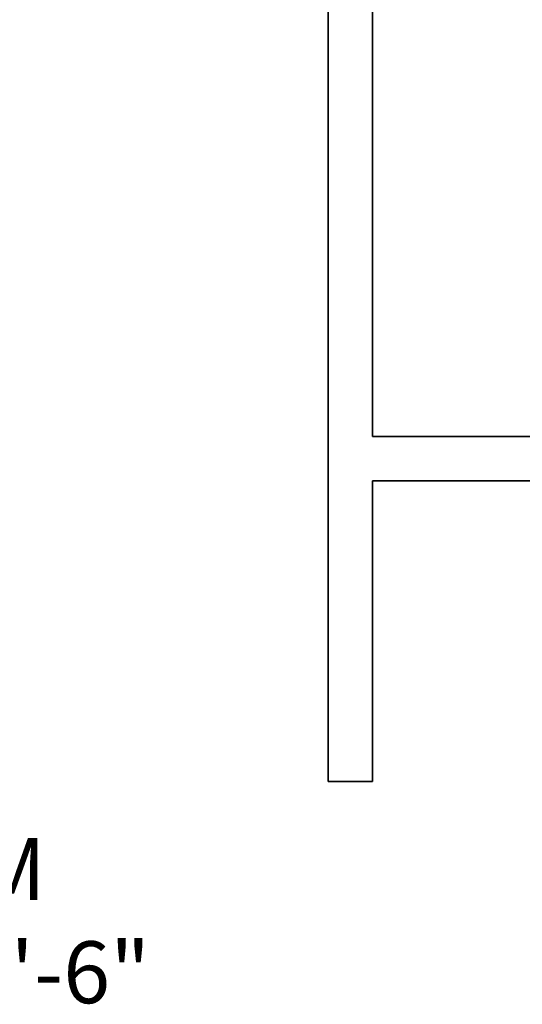
# Model space of a CAD drawing. Units: inches. Extents: x 3731 to 4318, y 1310 to 2388.
# Tile 39 of 57: x 3943 to 4000, y 2198 to 2310. Entities that reach past the tile are written whole.
import ezdxf

# ---------------------------------------------------------------- set-up
doc = ezdxf.new("R2010")
doc.units = ezdxf.units.IN
doc.layers.add('A-AREA-IDEN', color=7, linetype='Continuous', lineweight=18)
doc.layers.add('A-WALL', color=7, linetype='Continuous', lineweight=35)
doc.styles.get("Standard").update_dxf_attribs({"font": 'arial.ttf'})

msp = doc.modelspace()

# ---------------------------------------------------------------- linework, layer by layer
at = {"layer": 'A-WALL'}
for p, q in [((3983.21, 2338.38), (3983.21, 2262.38)), ((3978.21, 2333.38), (3978.21, 2223.38)), ((3983.21, 2262.38), (4103.21, 2262.38)), ((3983.21, 2257.38), (4103.21, 2257.38)), ((3983.21, 2257.38), (3983.21, 2223.38)), ((3978.21, 2223.38), (3983.21, 2223.38))]:
    msp.add_line(p, q, dxfattribs=at)

# ---------------------------------------------------------------- texts
at = {"layer": 'A-AREA-IDEN', "insert": (3899.81, 2216.97), "char_height": 7, "attachment_point": 1}
msp.add_mtext_dynamic_manual_height_columns('BEDROOM\\P11\'-6"X12\'-6"', width=47.0437, gutter_width=12.5, heights=[0], dxfattribs=at)

doc.saveas('drawing.dxf')
